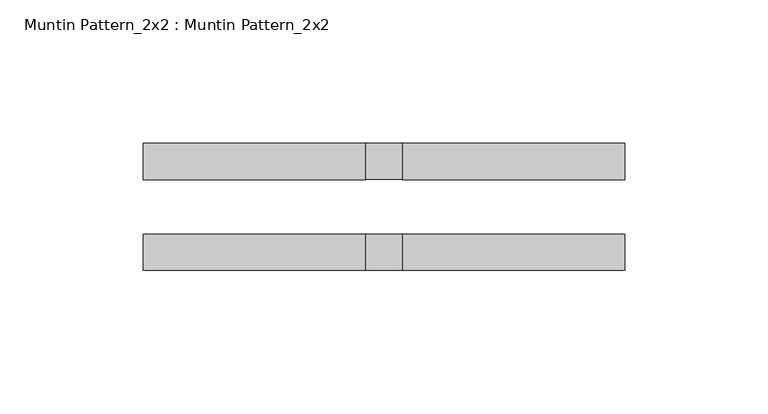
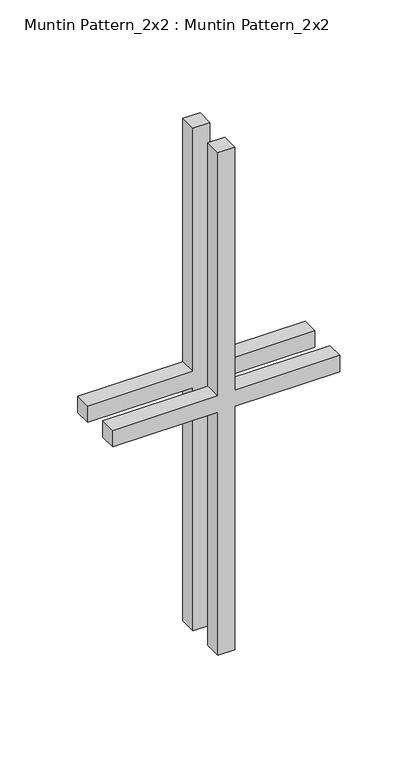
"""IFC4 building model written with IfcOpenShell, lengths in millimetres: proxy geometry, Muntin Pattern_2x2 : Muntin Pattern_2x2."""

from ifc_helpers import new_model, si_unit, frame, origin, place, context, project, spatial, polyline, outline, extrude, source, transform, mapped, element, save


def muntin_pattern_2x2_muntin_pattern_2x2_653c8599(model_context):
    return source(origin(), model_context, "Body", "SweptSolid", [
        extrude(outline(polyline([(203.2, -6.35), (203.2, -84.1375), (190.5, -84.1375), (190.5, -6.35), (0.0, -6.35), (0.0, 6.35), (190.5, 6.35), (190.5, 84.1375), (203.2, 84.1375), (203.2, 6.35), (393.7, 6.35), (393.7, -6.35), (203.2, -6.35)])), frame((0.0, 9.525, 0.0), z_axis=(0.0, 1.0, 0.0), x_axis=(0.0, 0.0, 1.0)), (0.0, 0.0, 1.0), 12.7),
        extrude(outline(polyline([(203.2, -6.35), (203.2, -84.1375), (190.5, -84.1375), (190.5, -6.35), (0.0, -6.35), (0.0, 6.35), (190.5, 6.35), (190.5, 84.1375), (203.2, 84.1375), (203.2, 6.35), (393.7, 6.35), (393.7, -6.35), (203.2, -6.35)])), frame((0.0, -22.225, 0.0), z_axis=(0.0, 1.0, 0.0), x_axis=(0.0, 0.0, 1.0)), (0.0, 0.0, 1.0), 12.7),
    ])


if __name__ == "__main__":
    model = new_model("IFC4")
    model_context = context("Model", 3, world=origin())
    ifc_project = project(units=[si_unit("LENGTHUNIT", "METRE", prefix="MILLI")], contexts=[model_context])
    site = spatial("IfcSite", under=ifc_project)
    building = spatial("IfcBuilding", under=site)
    placement = place(None, origin())
    muntin_pattern_2x2_muntin_pattern_2x2_shape = muntin_pattern_2x2_muntin_pattern_2x2_653c8599(model_context)
    element("IfcBuildingElementProxy", 1, Name="Muntin Pattern_2x2 : Muntin Pattern_2x2", ObjectType="Muntin Pattern_2x2 : Muntin Pattern_2x2", at=placement, inside=building, context=model_context, shape_type="MappedRepresentation", body=[
        mapped(muntin_pattern_2x2_muntin_pattern_2x2_shape, transform((0.0, 0.0, 0.0), x_axis=(1.0, 0.0, 0.0), y_axis=(0.0, 1.0, 0.0), z_axis=(0.0, 0.0, 1.0))),
    ])
    save(model, "model.ifc")

# Revit data of these elements
# Type "Muntin Pattern_2x2 : Muntin Pattern_2x2"
#   Width [instance default] = 4' - 0"
#   Thickness = 0' - 0 1/2"
#   Height [instance default] = 4' - 0"
#   Distance = 0' - 0 3/4"
#   Interior Material [instance default] = none
#   Exterior Material [instance default] = none
#   Default Elevation = 0
# Element 1 (IfcBuildingElementProxy, "Muntin Pattern_2x2 : Muntin Pattern_2x2")
#   Width = 0' - 6 5/8"
#   Height = 1' - 3 1/2"
#   Interior Material = Wood - Stained
#   Exterior Material = Clad - White
#   Materials on its faces: "Clad - White", "Wood - Stained"
# Materials
#   "Clad - White": class "Wood", colour RGB 242 242 238, transparency 0, Cost = 0
#   "Wood - Stained": class "Wood", colour RGB 224 178 126, transparency 0, Cost = 0
